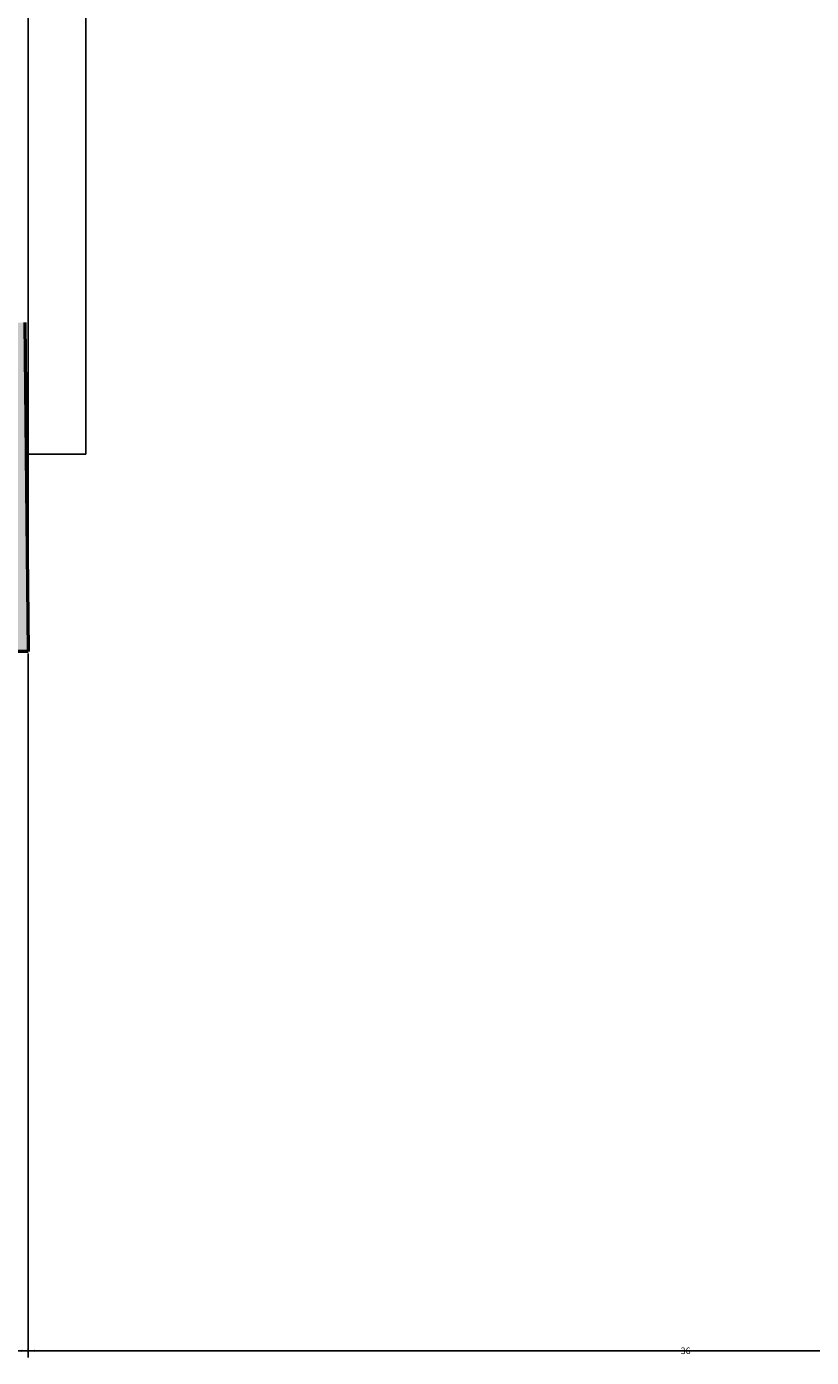
# Model space of a CAD drawing. Units: inches. Extents: x 2307 to 2544, y 2171 to 2540.
# Tile 7 of 52: x 2434 to 2455, y 2171 to 2208. Entities that reach past the tile are written whole.
import ezdxf

# ---------------------------------------------------------------- set-up
doc = ezdxf.new("R2010")
doc.units = ezdxf.units.IN
for name, color, linetype, lineweight in [('A-ANNO-DIMS', 2, 'Continuous', 18), ('A-DOOR', 3, 'Continuous', 25), ('A-WALL', 7, 'Continuous', 50)]:
    doc.layers.add(name, color=color, linetype=linetype, lineweight=lineweight)
doc.layers.add('A-WALL-PATT', color=18, linetype='Continuous', lineweight=13, true_color=0x000000)
doc.styles.get("Standard").update_dxf_attribs({"font": 'arial.ttf'})
doc.dimstyles.get("Standard").update_dxf_attribs({"dimtxt": 0.18, "dimasz": 0.18, "dimexe": 0.18, "dimexo": 0.0625, "dimgap": 0.09, "dimtad": 0, "dimtih": 1, "dimtoh": 1, "dimdec": 4, "dimzin": 0, "dimdsep": 46, "dimtxsty": 'Standard', "dimcen": 0.09, "dimadec": 0, "dimazin": 0, "dimtfac": 1, "dimtdec": 4, "dimtofl": 0, "dimtmove": 0, "dimatfit": 3, "dimfxl": 1, "dimtolj": 1, "dimtzin": 0, "dimarcsym": 0})

# ---------------------------------------------------------------- blocks, each defined once
blk = doc.blocks.new('*U13')
blk.add_line((0, 0), (0, -6))
blk.add_lwpolyline([(0, 0), (0, 40), (1.75, 40), (1.75, 0)], close=True)
blk.add_arc((0, 0), 40, 0, 90)
blk = doc.blocks.new('*D36')
at = {"layer": 'A-ANNO-DIMS', "color": 0, "lineweight": -2, "transparency": 16777216}
for p, q in [((2326.696, 2190.447), (2326.696, 2171.18)), ((2524.696, 2190.447), (2524.696, 2171.18)), ((2326.876, 2171.36), (2425.415, 2171.36)), ((2524.516, 2171.36), (2425.976, 2171.36))]:
    blk.add_line(p, q, dxfattribs=at)
at = {"layer": 'A-ANNO-DIMS', "color": 0, "transparency": 16777216}
for points in [[(2326.876, 2171.39), (2326.876, 2171.33), (2326.696, 2171.36)], [(2524.516, 2171.39), (2524.516, 2171.33), (2524.696, 2171.36)]]:
    blk.add_solid(points, dxfattribs=at)
at = {"layer": 'Defpoints', "color": 0, "transparency": 16777216}
for p in [(2326.696, 2190.51), (2524.696, 2190.51), (2524.696, 2171.36)]:
    blk.add_point(p, dxfattribs=at)
at = {"layer": 'A-ANNO-DIMS', "color": 0, "transparency": 16777216, "insert": (2425.696, 2171.36), "char_height": 0.18, "attachment_point": 5}
blk.add_mtext('\\A1;198', dxfattribs=at)
blk = doc.blocks.new('*D38')
at = {"layer": 'A-ANNO-DIMS', "color": 0, "lineweight": -2, "transparency": 16777216}
for p, q in [((2415.642, 2190.447), (2415.642, 2171.18)), ((2433.783, 2190.447), (2433.783, 2171.18)), ((2415.822, 2171.36), (2424.328, 2171.36)), ((2433.603, 2171.36), (2425.098, 2171.36))]:
    blk.add_line(p, q, dxfattribs=at)
at = {"layer": 'A-ANNO-DIMS', "color": 0, "transparency": 16777216}
for points in [[(2415.822, 2171.39), (2415.822, 2171.33), (2415.642, 2171.36)], [(2433.603, 2171.39), (2433.603, 2171.33), (2433.783, 2171.36)]]:
    blk.add_solid(points, dxfattribs=at)
at = {"layer": 'Defpoints', "color": 0, "transparency": 16777216}
for p in [(2415.642, 2190.51), (2433.783, 2190.51), (2433.783, 2171.36)]:
    blk.add_point(p, dxfattribs=at)
at = {"layer": 'A-ANNO-DIMS', "color": 0, "transparency": 16777216, "insert": (2424.713, 2171.36), "char_height": 0.18, "attachment_point": 5}
blk.add_mtext('\\A1;18.14', dxfattribs=at)
blk = doc.blocks.new('*D40')
at = {"layer": 'A-ANNO-DIMS', "color": 0, "lineweight": -2, "transparency": 16777216}
for p, q in [((2433.783, 2190.447), (2433.783, 2171.18)), ((2469.783, 2190.447), (2469.783, 2171.18)), ((2433.963, 2171.36), (2451.564, 2171.36)), ((2469.603, 2171.36), (2452.002, 2171.36))]:
    blk.add_line(p, q, dxfattribs=at)
at = {"layer": 'A-ANNO-DIMS', "color": 0, "transparency": 16777216}
for points in [[(2433.963, 2171.39), (2433.963, 2171.33), (2433.783, 2171.36)], [(2469.603, 2171.39), (2469.603, 2171.33), (2469.783, 2171.36)]]:
    blk.add_solid(points, dxfattribs=at)
at = {"layer": 'Defpoints', "color": 0, "transparency": 16777216}
for p in [(2433.783, 2190.51), (2469.783, 2190.51), (2469.783, 2171.36)]:
    blk.add_point(p, dxfattribs=at)
at = {"layer": 'A-ANNO-DIMS', "color": 0, "transparency": 16777216, "insert": (2451.783, 2171.36), "char_height": 0.18, "attachment_point": 5}
blk.add_mtext('\\A1;36', dxfattribs=at)

msp = doc.modelspace()

# ---------------------------------------------------------------- hatches: boundary and pattern name
at = {"layer": 'A-WALL-PATT'}
h = msp.add_hatch(color=256, dxfattribs=at)
h.dxf.hatch_style = 1
h.paths.add_polyline_path([(2433.6935, 2199.5096), (2415.6423, 2199.5096), (2415.6423, 2190.5096), (2433.7832, 2190.5096)], flags=17)
h.paths.add_polyline_path([(2367.6423, 2199.5096), (2335.6958, 2199.5096), (2335.6958, 2307.3983), (2326.6958, 2307.3983), (2326.6958, 2190.5096), (2367.6423, 2190.5096)])
h.paths.add_polyline_path([(2524.6958, 2520.5096), (2496.7832, 2520.5096), (2496.7832, 2515.5149), (2472.7832, 2515.5149), (2472.7832, 2520.5096), (2415.4028, 2520.5096), (2415.4028, 2511.5096), (2451.6958, 2511.5096), (2451.6958, 2439.5096), (2451.6958, 2391.5096), (2445.6958, 2391.5096), (2445.6958, 2387.5096), (2455.6958, 2387.5096), (2455.6958, 2435.5096), (2461.6958, 2435.5096), (2461.6958, 2439.5096), (2455.6958, 2439.5096), (2455.6958, 2511.5096), (2515.6958, 2511.5096), (2515.6958, 2439.5096), (2491.6958, 2439.5096), (2491.6958, 2435.5096), (2515.6958, 2435.5096), (2515.6958, 2319.5096), (2451.6958, 2319.5096), (2451.6958, 2281.5096), (2481.6958, 2281.5096), (2481.6958, 2225.5096), (2485.6958, 2225.5096), (2485.6958, 2285.5096), (2455.6958, 2285.5096), (2455.6958, 2315.5096), (2515.6958, 2315.5096), (2515.6958, 2199.5096), (2469.6952, 2199.5096), (2469.785, 2190.5096), (2524.6958, 2190.5096)])

# ---------------------------------------------------------------- linework, layer by layer
at = {"layer": 'A-WALL'}
msp.add_line((2433.6935, 2199.5096), (2433.7832, 2190.5096), dxfattribs=at)
msp.add_lwpolyline([(2433.7832, 2190.5096), (2326.6958, 2190.5096), (2326.6958, 2520.5096), (2524.6958, 2520.5096), (2524.6958, 2190.5096), (2469.785, 2190.5096)], dxfattribs=at)

# ---------------------------------------------------------------- block references
at = {"layer": 'A-DOOR', "xscale": 0.9, "yscale": 0.9, "zscale": 0.9}
msp.add_blockref('*U13', (2433.7832, 2195.9096), dxfattribs=at)

# ---------------------------------------------------------------- dimensions: what is measured, and where the dimension line sits
at = {"layer": 'A-ANNO-DIMS'}
for base, p1, p2, override, picture, middle in [((2524.6958, 2171.3596), (2326.6958, 2190.5096), (2524.6958, 2190.5096), {"dimdec": 0, "dimlfac": 1, "dimrnd": 0, "dimzin": 0, "dimdsep": 46, "dimlunit": 2}, '*D36', (2425.6958, 2171.3596)), ((2433.7832, 2171.3596), (2415.6423, 2190.5096), (2433.7832, 2190.5096), {"dimdec": 2, "dimlfac": 1, "dimrnd": 0, "dimzin": 0, "dimdsep": 46, "dimlunit": 2}, '*D38', (2424.7128, 2171.3596)), ((2469.7832, 2171.3596), (2433.7832, 2190.5096), (2469.7832, 2190.5096), {"dimdec": 0, "dimlfac": 1, "dimrnd": 0, "dimzin": 0, "dimdsep": 46, "dimlunit": 2}, '*D40', (2451.7832, 2171.3596))]:
    dim = msp.add_linear_dim(base=base, p1=p1, p2=p2, dimstyle='Standard', override=override, dxfattribs=at)
    dim.commit()
    dim.dimension.update_dxf_attribs({"geometry": picture, "text_midpoint": middle})

doc.saveas('drawing.dxf')
